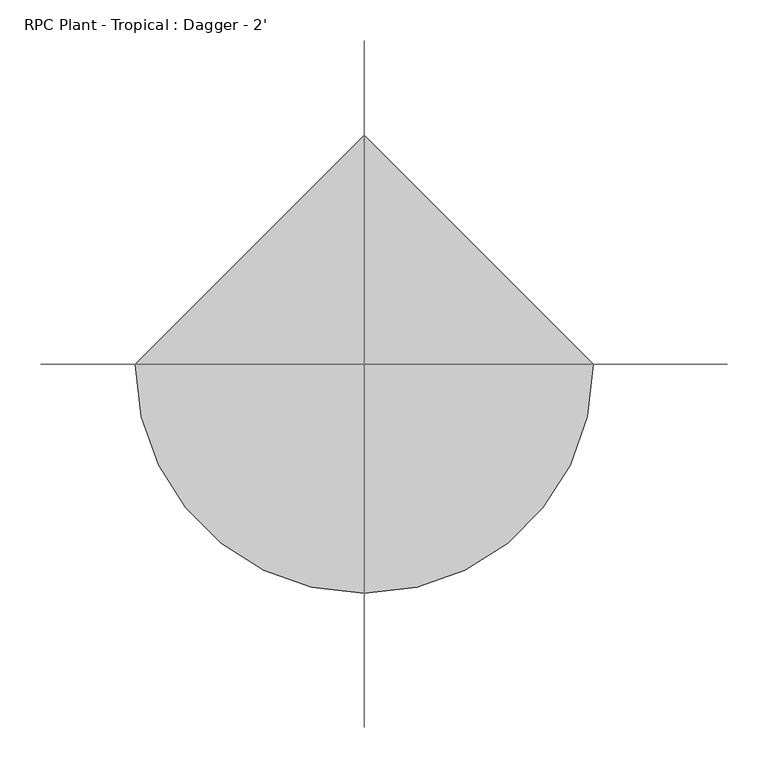
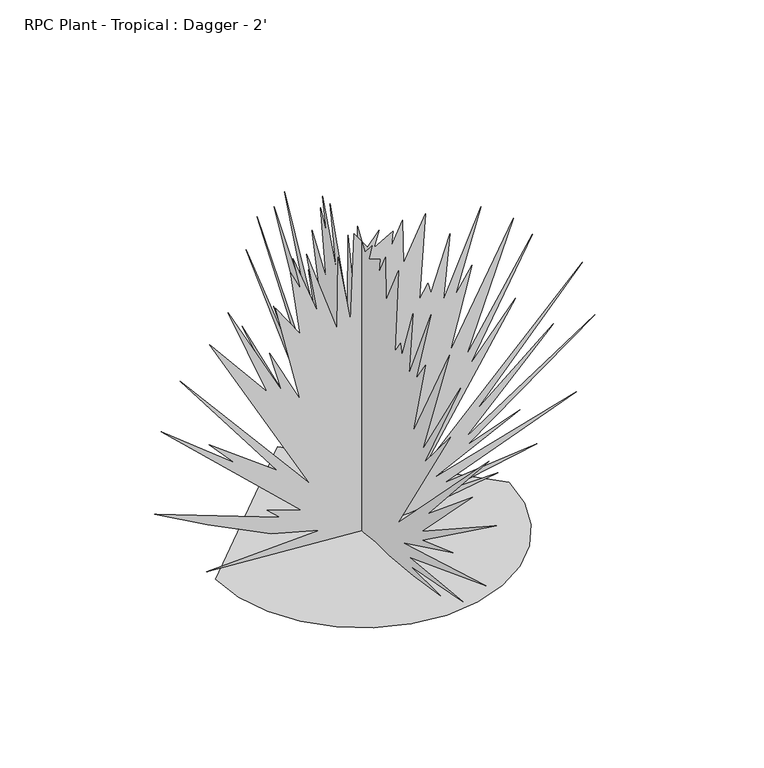
"""IFC4 building model written with IfcOpenShell, lengths in millimetres: geographic element geometry, RPC Plant - Tropical : Dagger - 2'."""

from ifc_helpers import new_model, si_unit, origin, place, context, project, spatial, triangles, source, transform, mapped, element, save


def rpc_plant_tropical_dagger_2_80c14bd7(model_context):
    return source(origin(), model_context, "Body", "Tessellation", [
        triangles([(-0.0169483, -5.816808, 0.0), (-0.0169288, 298.9836399, 21.1666745), (-0.0169413, 81.6722405, 29.6334406), (-0.0169342, 174.805482, 55.033464), (-0.0169232, 297.5713896, 117.1222841), (-0.0169138, 399.1714926, 173.5667131), (-0.0169336, 157.8723041, 83.2556831), (-0.0169307, 183.2723162, 105.8335019), (-0.016936, 116.9500744, 83.2556831), (-0.0169048, 386.4714684, 337.2563765), (-0.0169199, 245.3611499, 224.3667555), (-0.0169138, 294.7494507, 277.9879738), (-0.0169274, 163.5166906, 180.6223326), (-0.0169017, 349.7836641, 426.1564734), (-0.0169339, 101.427866, 132.6444926), (-0.0169017, 293.339762, 481.1881433), (-0.0169163, 183.2723162, 347.1344436), (-0.0169007, 258.0616646, 533.400436), (-0.0169184, 155.0501108, 340.0783336), (-0.0169121, 177.6279296, 423.3345162), (-0.0169223, 119.7722677, 309.0344436), (-0.0169075, 166.3388839, 510.8223447), (-0.0169144, 119.7722677, 443.088107), (-0.0169055, 138.1166785, 572.9127045), (-0.016909, 118.3610439, 533.400436), (-0.0169042, 132.4722829, 599.7224052), (-0.0169145, 85.9054123, 475.5442655), (-0.0169058, 107.0722617, 599.7224052), (-0.0169196, 47.8056303, 427.566162), (-0.016911, 46.3944065, 572.9127045), (-0.0169207, 22.4054592, 434.622272), (-0.0169106, 15.349867, 609.6005087), (-0.0169144, -10.050077, 572.9127045), (-0.0169141, -32.6278504, 599.7224052), (-0.0169154, -22.7501125, 567.2662831), (-0.0169164, -59.4390954, 588.4346495), (-0.0169179, -56.6168975, 560.2126802), (-0.0169166, -77.7834971, 603.9565945), (-0.0169218, -79.1947209, 516.4662226), (-0.0169192, -121.52792, 602.5443624), (-0.0169287, -110.2391378, 431.8003512), (-0.0169282, -127.17257, 458.6125955), (-0.0169297, -132.8169566, 437.4442291), (-0.0169255, -169.5057691, 544.6881918), (-0.0169325, -156.8057631, 414.8661378), (-0.0169271, -228.7723914, 578.5565824), (-0.0169337, -179.3835819, 417.6880949), (-0.0169328, -211.8392135, 465.6661983), (-0.0169399, -169.5057691, 304.8002543), (-0.0169334, -290.8607164, 533.400436), (-0.0169428, -200.550186, 286.4563522), (-0.0169383, -327.5510459, 488.2442533), (-0.0169445, -207.6057873, 265.2879677), (-0.0169435, -295.0948874, 369.7125349), (-0.0169498, -120.1169505, 88.9000696), (-0.0169494, -423.5072528, 397.9345041), (-0.016951, -218.8948329, 167.9223265), (-0.0169525, -368.473003, 292.1002301), (-0.0169526, -199.1392074, 119.9444865), (-0.0169578, -447.4950328, 282.222163), (-0.0169538, -201.9614007, 103.0113086), (-0.0169577, -303.5607224, 139.700112), (-0.0169526, -137.0501284, 59.2666313), (-0.0169642, -412.2169172, 138.2888882), (-0.0169548, -158.2169778, 42.3334534), (-0.0169644, -336.0168809, 59.2666313), (-0.0169559, -159.6279563, 25.4000212), (-0.0169619, -261.2290403, 26.811245), (-0.0169573, -170.9169838, 12.7000106), (-0.0169529, -89.0722793, 4.2333197), (-0.0169503, -43.9168869, 4.2333197), (-282.2577168, 0.0, 0.0937388), (-274.7951999, -64.6747996, 0.0937388), (-253.5445348, -124.0684354, 0.0937388), (-220.2049637, -176.4790898, 0.0937388), (-176.4790898, -220.2049637, 0.0937388), (-124.0684354, -253.5445348, 0.0937388), (-64.6747996, -274.7951999, 0.0937388), (1.23e-05, -282.2577168, 0.0937388), (64.6747996, -274.7951999, 0.0937388), (124.0684354, -253.5445348, 0.0937388), (176.4790898, -220.2049637, 0.0937388), (220.2049637, -176.4790898, 0.0937388), (253.5445348, -124.0684354, 0.0937388), (274.7951999, -64.6747996, 0.0937388), (282.2577168, 2.47e-05, 0.0937388), (-3.7e-05, 282.2577168, 0.0937388), (5.816808, 0.0169479, 0.0), (-298.9836399, 0.0169466, 21.1666745), (-81.6722405, 0.0169461, 29.6334406), (-174.8057363, 0.0169446, 55.033464), (-297.5713896, 0.0169409, 117.1222841), (-399.1714926, 0.0169375, 173.5667131), (-157.8723041, 0.016943, 83.2556831), (-183.2723162, 0.0169416, 105.8335019), (-116.9500744, 0.016943, 83.2556831), (-386.4714684, 0.0169278, 337.2563765), (-245.3611499, 0.0169345, 224.3667555), (-294.7494507, 0.0169313, 277.9879738), (-163.5166906, 0.0169371, 180.6223326), (-349.7836641, 0.0169225, 426.1564734), (-101.427866, 0.01694, 132.6444926), (-293.339762, 0.0169192, 481.1881433), (-183.2723162, 0.0169272, 347.1344436), (-258.0616646, 0.0169161, 533.400436), (-155.0501108, 0.0169277, 340.0783336), (-177.6279296, 0.0169227, 423.3345162), (-119.7722677, 0.0169295, 309.0344436), (-166.3388839, 0.0169175, 510.8223447), (-119.7722677, 0.0169215, 443.088107), (-138.1166785, 0.0169138, 572.9127045), (-118.3610439, 0.0169161, 533.400436), (-132.4722829, 0.0169121, 599.7224052), (-85.9054123, 0.0169196, 475.5442655), (-107.0722617, 0.0169121, 599.7224052), (-47.8056303, 0.0169224, 427.566162), (-46.3944065, 0.0169138, 572.9127045), (-22.4054592, 0.016922, 434.622272), (-15.3498931, 0.0169116, 609.6005087), (10.0501019, 0.0169138, 572.9127045), (32.6278504, 0.0169121, 599.7224052), (22.7501125, 0.0169141, 567.2662831), (59.4390954, 0.0169129, 588.4346495), (56.6168975, 0.0169145, 560.2126802), (77.7834971, 0.0169119, 603.9565945), (79.1947209, 0.0169171, 516.4662226), (121.52792, 0.016912, 602.5443624), (110.2391378, 0.0169222, 431.8003512), (127.17257, 0.0169206, 458.6125955), (132.8169566, 0.0169218, 437.4442291), (169.5057691, 0.0169154, 544.6881918), (156.8057631, 0.0169232, 414.8661378), (228.7723914, 0.0169134, 578.5565824), (179.3835819, 0.016923, 417.6880949), (211.8392135, 0.0169201, 465.6661983), (169.5057691, 0.0169297, 304.8002543), (290.8607164, 0.0169161, 533.400436), (200.550186, 0.0169308, 286.4563522), (327.5510459, 0.0169188, 488.2442533), (207.6057873, 0.0169321, 265.2879677), (295.0948874, 0.0169259, 369.7125349), (120.1169505, 0.0169426, 88.9000696), (423.5072528, 0.0169242, 397.9345041), (218.8948329, 0.0169379, 167.9223265), (368.473003, 0.0169305, 292.1002301), (199.1392074, 0.0169408, 119.9444865), (447.4950328, 0.0169311, 282.222163), (201.9614007, 0.0169418, 103.0113086), (303.5607224, 0.0169396, 139.700112), (137.0501284, 0.0169444, 59.2666313), (412.2169172, 0.0169397, 138.2888882), (158.2169778, 0.0169454, 42.3334534), (336.0168809, 0.0169444, 59.2666313), (159.6279563, 0.0169464, 25.4000212), (261.2290403, 0.0169463, 26.811245), (170.9169838, 0.0169471, 12.7000106), (89.0722793, 0.0169477, 4.2333197), (43.9168869, 0.0169477, 4.2333197)], [[68, 67, 69], [69, 67, 70], [64, 63, 65], [62, 61, 63], [58, 57, 59], [56, 55, 57], [57, 55, 59], [52, 51, 53], [50, 49, 51], [48, 47, 49], [46, 45, 47], [47, 45, 49], [40, 39, 41], [36, 35, 37], [34, 33, 35], [28, 27, 29], [26, 25, 27], [24, 23, 25], [22, 21, 23], [20, 19, 21], [16, 15, 17], [12, 11, 13], [10, 9, 11], [11, 9, 13], [8, 7, 9], [2, 1, 3], [66, 65, 67], [67, 65, 70], [65, 63, 70], [60, 59, 61], [61, 59, 63], [59, 55, 63], [63, 55, 70], [54, 53, 55], [53, 51, 55], [51, 49, 55], [49, 45, 55], [44, 43, 45], [45, 43, 55], [43, 42, 55], [42, 41, 55], [55, 41, 70], [41, 39, 70], [70, 39, 71], [39, 38, 71], [38, 37, 71], [37, 35, 71], [71, 35, 1], [35, 33, 1], [33, 32, 1], [18, 17, 19], [17, 15, 19], [19, 15, 21], [14, 13, 15], [13, 9, 15], [6, 5, 7], [5, 4, 7], [4, 3, 7], [7, 3, 9], [9, 3, 15], [21, 15, 23], [23, 15, 25], [25, 15, 27], [15, 3, 27], [27, 3, 29], [3, 1, 29], [29, 1, 30], [30, 1, 31], [1, 32, 31], [86, 87, 72], [85, 86, 72], [85, 72, 73], [84, 85, 73], [84, 73, 74], [84, 74, 75], [83, 84, 75], [82, 83, 75], [82, 75, 76], [82, 76, 77], [82, 77, 78], [82, 78, 79], [82, 79, 80], [82, 80, 81], [154, 155, 156], [154, 156, 157], [150, 151, 152], [148, 149, 150], [144, 145, 146], [142, 143, 144], [142, 144, 146], [138, 139, 140], [136, 137, 138], [134, 135, 136], [132, 133, 134], [132, 134, 136], [126, 127, 128], [122, 123, 124], [120, 121, 122], [114, 115, 116], [112, 113, 114], [110, 111, 112], [108, 109, 110], [106, 107, 108], [102, 103, 104], [98, 99, 100], [96, 97, 98], [96, 98, 100], [94, 95, 96], [88, 89, 90], [152, 153, 154], [152, 154, 157], [150, 152, 157], [146, 147, 148], [146, 148, 150], [142, 146, 150], [142, 150, 157], [140, 141, 142], [138, 140, 142], [136, 138, 142], [132, 136, 142], [130, 131, 132], [130, 132, 142], [129, 130, 142], [128, 129, 142], [128, 142, 157], [126, 128, 157], [126, 157, 158], [125, 126, 158], [124, 125, 158], [122, 124, 158], [122, 158, 88], [120, 122, 88], [119, 120, 88], [104, 105, 106], [102, 104, 106], [102, 106, 108], [100, 101, 102], [96, 100, 102], [92, 93, 94], [91, 92, 94], [90, 91, 94], [90, 94, 96], [90, 96, 102], [102, 108, 110], [102, 110, 112], [102, 112, 114], [90, 102, 114], [90, 114, 116], [88, 90, 116], [88, 116, 117], [88, 117, 118], [119, 88, 118]], closed=False),
    ])


if __name__ == "__main__":
    model = new_model("IFC4")
    model_context = context("Model", 3, world=origin())
    ifc_project = project(units=[si_unit("LENGTHUNIT", "METRE", prefix="MILLI")], contexts=[model_context])
    site = spatial("IfcSite", under=ifc_project)
    building = spatial("IfcBuilding", under=site)
    placement = place(None, origin())
    rpc_plant_tropical_dagger_2_shape = rpc_plant_tropical_dagger_2_80c14bd7(model_context)
    element("IfcGeographicElement", 1, ObjectType="RPC Plant - Tropical : Dagger - 2'", at=placement, inside=building, context=model_context, shape_type="MappedRepresentation", body=[
        mapped(rpc_plant_tropical_dagger_2_shape, transform((0.0, 0.0, 0.0), x_axis=(1.0, 0.0, 0.0), y_axis=(0.0, 1.0, 0.0), z_axis=(0.0, 0.0, 1.0))),
    ])
    save(model, "model.ifc")

# Revit data of these elements
# Type "RPC Plant - Tropical : Dagger - 2'"
#   built-in parameter 1005198 = "{2, 15},{39, RPC-16-G3A7-NEG0-UH6H-J000-ST1L-LVER-AU},{1, 0},{1, 0},{2, 35},{1, 8},{5, Color},{1, 0},{1, 0},{3, 0.8},{3, 0.8},{3, 0.8},{1, 8},{7, BBoxMin},{1, 0},{1, 0},{1, 0},{1, 0},{1, 0},{1, 8},{7, BBoxMax},{1, 0},{1, 0},{1, 0},{1, 0},{1, 0},{2, 11},{9, RPCTypeId},{1, 0},{1, 0},{39, RPC-16-G3A7-NEG0-UH6H-J000-ST1L-LVER-AU},{1, 6},{14, RPCPlantHeight},{1, 0},{1, 0},{1, 2},{2, 11},{7, keyword},{1, 0},{1, 0},{55, :Geometry:RPC:Dagger:Yucca Recurvifolia:plant:tropical.},{2, 11},{8, category},{1, 0},{1, 0},{17, :Plants [General]},{2, 11},{12, LocalizedUID},{1, 0},{1, 0},{6, Dagger},{2, 14},{6, Height},{1, 0},{1, 0},{1, 2},{1, 2},{16, Cast Reflections},{1, 0},{1, 0},{1, 0},{1, 2},{12, Cast Shadows},{1, 0},{1, 0},{1, 1},{1, 2},{9, Lock View},{1, 0},{1, 0},{1, 0},{1, 4},{5, ViewC},{1, 0},{1, 0},{1, 0},{2, 11},{20, AdvancedUIDefinition},{1, 0},{1, 0},{0, },{2, 11},{10, AssetLibID},{1, 0},{1, 0},{36, 4D3F6E72-3F99-4203-98E9-AF80B3C7A7A4},{2, 11},{10, BaseSchema},{1, 0},{1, 0},{9, RPCSchema},{2, 11},{12, ExchangeGUID},{1, 0},{1, 0},{0, },{1, 2},{6, Hidden},{1, 0},{1, 0},{1, 0},{1, 4},{11, RPCCategory},{1, 0},{1, 0},{1, 0},{2, 11},{8, RPCImage},{1, 0},{1, 0},{0, },{1, 4},{13, SchemaVersion},{1, 0},{1, 0},{1, 4},{2, 11},{12, UIDefinition},{1, 0},{1, 0},{0, },{2, 11},{6, UIName},{1, 0},{1, 0},{39, RPC-16-G3A7-NEG0-UH6H-J000-ST1L-LVER-AU},{2, 11},{11, VersionGUID},{1, 0},{1, 0},{9, RPCSchema},{2, 11},{9, assettype},{1, 0},{1, 0},{11, RPCGeometry},{2, 11},{11, description},{1, 0},{1, 0},{0, },{2, 11},{9, localname},{1, 0},{1, 0},{3, RPC},{2, 11},{9, localtype},{1, 0},{1, 0},{3, RPC},{1, 4},{8, revision},{1, 0},{1, 0},{1, 1},{2, 11},{9, thumbnail},{1, 0},{1, 0},{0, },{1, 4},{7, version},{1, 0},{1, 0},{1, 1},{1, 2},{20, RPC_Cast Reflections},{1, 0},{1, 0},{1, 1},{1, 2},{16, RPC_Cast Shadows},{1, 0},{1, 0},{1, 1},{1, 2},{13, RPC_Lock View},{1, 0},{1, 0},{1, 0},{1, 4},{9, RPC_ViewC},{1, 0},{1, 0},{1, 0},{21, assetlibrary_base.fbx},{1, 5},"
#   built-in parameter 1005195 = "RPC-16-G3A7-NEG0-UH6H-J000-ST1L-LVER-AU"
#   Type Comments = "Dagger"
#   Assembly Code = "G2050500"
#   Height = 2' - 0"
#   Default Elevation = 0
